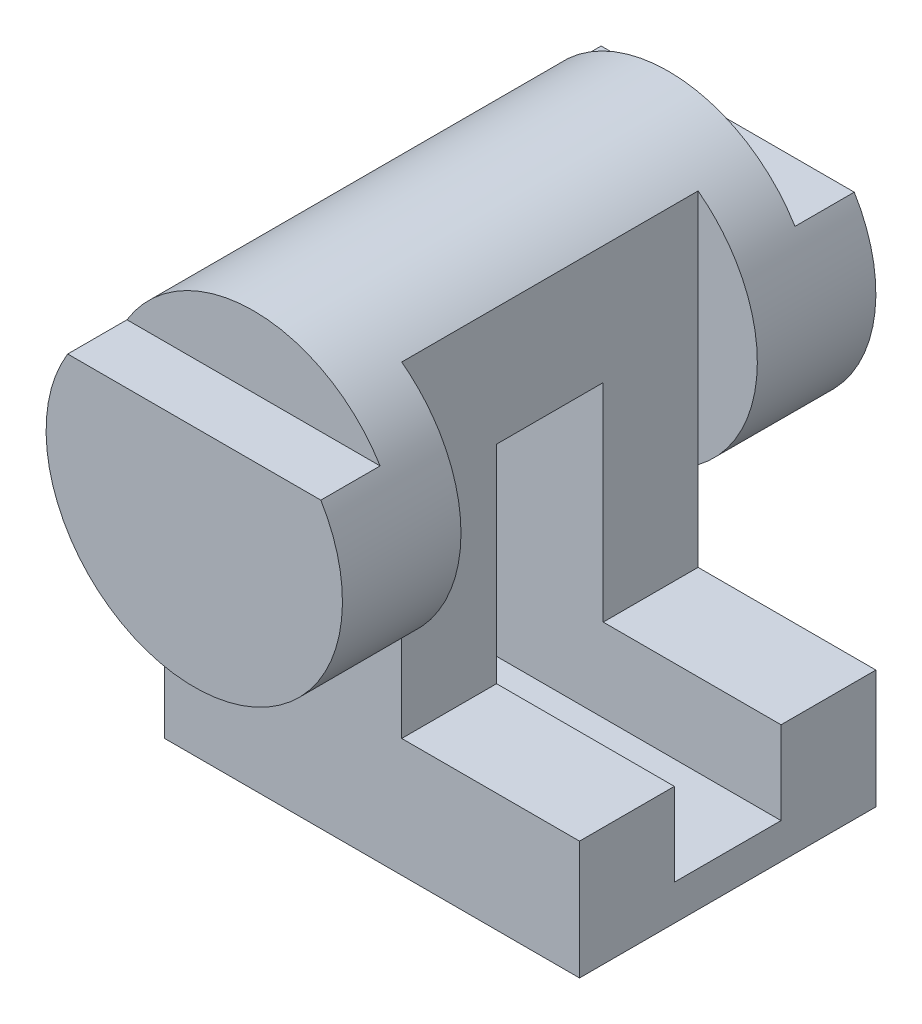
ISO-10303-21;
HEADER;
FILE_DESCRIPTION(('STEP AP214'),'2;1');
FILE_NAME('part.step','',(''),(''),'','','');
FILE_SCHEMA(('AUTOMOTIVE_DESIGN { 1 0 10303 214 1 1 1 1 }'));
ENDSEC;
DATA;
#1=APPLICATION_CONTEXT('core data for automotive mechanical design processes');
#2=APPLICATION_PROTOCOL_DEFINITION('international standard','automotive_design',2000,#1);
#3=PRODUCT_CONTEXT('',#1,'mechanical');
#4=PRODUCT('Part','Part','',(#3));
#5=PRODUCT_RELATED_PRODUCT_CATEGORY('part','',(#4));
#6=PRODUCT_DEFINITION_FORMATION('','',#4);
#7=PRODUCT_DEFINITION_CONTEXT('part definition',#1,'design');
#8=PRODUCT_DEFINITION('design','',#6,#7);
#9=PRODUCT_DEFINITION_SHAPE('','',#8);
#10=(LENGTH_UNIT() NAMED_UNIT(*) SI_UNIT(.MILLI.,.METRE.));
#11=(NAMED_UNIT(*) PLANE_ANGLE_UNIT() SI_UNIT($,.RADIAN.));
#12=(NAMED_UNIT(*) SI_UNIT($,.STERADIAN.) SOLID_ANGLE_UNIT());
#13=UNCERTAINTY_MEASURE_WITH_UNIT(LENGTH_MEASURE(1.E-05),#10,'distance_accuracy_value','');
#14=(GEOMETRIC_REPRESENTATION_CONTEXT(3) GLOBAL_UNCERTAINTY_ASSIGNED_CONTEXT((#13)) GLOBAL_UNIT_ASSIGNED_CONTEXT((#10,
#11,#12)) REPRESENTATION_CONTEXT('',''));
#15=CARTESIAN_POINT('',(0.,0.,0.));
#16=DIRECTION('',(0.,0.,1.));
#17=DIRECTION('',(1.,0.,0.));
#18=AXIS2_PLACEMENT_3D('',#15,#16,#17);
#19=CARTESIAN_POINT('',(20.,0.,25.));
#20=DIRECTION('',(0.,0.,-1.));
#21=DIRECTION('',(-1.,0.,0.));
#22=AXIS2_PLACEMENT_3D('',#19,#20,#21);
#23=PLANE('',#22);
#24=CARTESIAN_POINT('',(-25.,55.,25.));
#25=DIRECTION('',(0.,0.,1.));
#26=DIRECTION('',(1.,0.,0.));
#27=AXIS2_PLACEMENT_3D('',#24,#25,#26);
#28=CIRCLE('',#27,25.);
#29=CARTESIAN_POINT('',(-50.,55.,25.));
#30=VERTEX_POINT('',#29);
#31=CARTESIAN_POINT('',(-10.,35.,25.));
#32=VERTEX_POINT('',#31);
#33=EDGE_CURVE('E57',#30,#32,#28,.T.);
#34=ORIENTED_EDGE('',*,*,#33,.F.);
#35=DIRECTION('',(0.,1.,0.));
#36=VECTOR('',#35,1.);
#37=CARTESIAN_POINT('',(-50.,0.,25.));
#38=LINE('',#37,#36);
#39=CARTESIAN_POINT('',(-50.,0.,25.));
#40=VERTEX_POINT('',#39);
#41=EDGE_CURVE('E246',#40,#30,#38,.T.);
#42=ORIENTED_EDGE('',*,*,#41,.F.);
#43=DIRECTION('',(-1.,0.,0.));
#44=VECTOR('',#43,1.);
#45=CARTESIAN_POINT('',(20.,0.,25.));
#46=LINE('',#45,#44);
#47=CARTESIAN_POINT('',(20.,0.,25.));
#48=VERTEX_POINT('',#47);
#49=EDGE_CURVE('E283',#48,#40,#46,.T.);
#50=ORIENTED_EDGE('',*,*,#49,.F.);
#51=DIRECTION('',(0.,-1.,0.));
#52=VECTOR('',#51,1.);
#53=CARTESIAN_POINT('',(20.,0.,25.));
#54=LINE('',#53,#52);
#55=CARTESIAN_POINT('',(20.,20.,25.));
#56=VERTEX_POINT('',#55);
#57=EDGE_CURVE('E261',#56,#48,#54,.T.);
#58=ORIENTED_EDGE('',*,*,#57,.F.);
#59=DIRECTION('',(-1.,0.,0.));
#60=VECTOR('',#59,1.);
#61=CARTESIAN_POINT('',(20.,20.,25.));
#62=LINE('',#61,#60);
#63=CARTESIAN_POINT('',(-10.,20.,25.));
#64=VERTEX_POINT('',#63);
#65=EDGE_CURVE('E284',#56,#64,#62,.T.);
#66=ORIENTED_EDGE('',*,*,#65,.T.);
#67=DIRECTION('',(0.,-1.,0.));
#68=VECTOR('',#67,1.);
#69=CARTESIAN_POINT('',(-10.,20.,25.));
#70=LINE('',#69,#68);
#71=EDGE_CURVE('E212',#32,#64,#70,.T.);
#72=ORIENTED_EDGE('',*,*,#71,.F.);
#73=EDGE_LOOP('',(#34,#42,#50,#58,#66,#72));
#74=FACE_BOUND('',#73,.T.);
#75=ADVANCED_FACE('F50',(#74),#23,.F.);
#76=CARTESIAN_POINT('',(20.,20.,-25.));
#77=DIRECTION('',(0.,0.,1.));
#78=DIRECTION('',(1.,0.,0.));
#79=AXIS2_PLACEMENT_3D('',#76,#77,#78);
#80=PLANE('',#79);
#81=CARTESIAN_POINT('',(-25.,55.,-25.));
#82=DIRECTION('',(0.,0.,-1.));
#83=DIRECTION('',(-1.,0.,0.));
#84=AXIS2_PLACEMENT_3D('',#81,#82,#83);
#85=CIRCLE('',#84,25.);
#86=CARTESIAN_POINT('',(-10.,35.,-25.));
#87=VERTEX_POINT('',#86);
#88=CARTESIAN_POINT('',(-50.,55.,-25.));
#89=VERTEX_POINT('',#88);
#90=EDGE_CURVE('E11',#87,#89,#85,.T.);
#91=ORIENTED_EDGE('',*,*,#90,.F.);
#92=DIRECTION('',(0.,1.,0.));
#93=VECTOR('',#92,1.);
#94=CARTESIAN_POINT('',(-10.,20.,-25.));
#95=LINE('',#94,#93);
#96=CARTESIAN_POINT('',(-10.,20.,-25.));
#97=VERTEX_POINT('',#96);
#98=EDGE_CURVE('E217',#97,#87,#95,.T.);
#99=ORIENTED_EDGE('',*,*,#98,.F.);
#100=DIRECTION('',(-1.,0.,0.));
#101=VECTOR('',#100,1.);
#102=CARTESIAN_POINT('',(20.,20.,-25.));
#103=LINE('',#102,#101);
#104=CARTESIAN_POINT('',(20.,20.,-25.));
#105=VERTEX_POINT('',#104);
#106=EDGE_CURVE('E276',#105,#97,#103,.T.);
#107=ORIENTED_EDGE('',*,*,#106,.F.);
#108=DIRECTION('',(0.,1.,0.));
#109=VECTOR('',#108,1.);
#110=CARTESIAN_POINT('',(20.,20.,-25.));
#111=LINE('',#110,#109);
#112=CARTESIAN_POINT('',(20.,0.,-25.));
#113=VERTEX_POINT('',#112);
#114=EDGE_CURVE('E264',#113,#105,#111,.T.);
#115=ORIENTED_EDGE('',*,*,#114,.F.);
#116=DIRECTION('',(-1.,0.,0.));
#117=VECTOR('',#116,1.);
#118=CARTESIAN_POINT('',(20.,0.,-25.));
#119=LINE('',#118,#117);
#120=CARTESIAN_POINT('',(-50.,0.,-25.));
#121=VERTEX_POINT('',#120);
#122=EDGE_CURVE('E281',#113,#121,#119,.T.);
#123=ORIENTED_EDGE('',*,*,#122,.T.);
#124=DIRECTION('',(0.,1.,0.));
#125=VECTOR('',#124,1.);
#126=CARTESIAN_POINT('',(-50.,0.,-25.));
#127=LINE('',#126,#125);
#128=EDGE_CURVE('E241',#121,#89,#127,.T.);
#129=ORIENTED_EDGE('',*,*,#128,.T.);
#130=EDGE_LOOP('',(#91,#99,#107,#115,#123,#129));
#131=FACE_BOUND('',#130,.T.);
#132=ADVANCED_FACE('F332',(#131),#80,.F.);
#133=CARTESIAN_POINT('',(20.,20.,9.));
#134=DIRECTION('',(0.,0.,1.));
#135=DIRECTION('',(0.,-1.,0.));
#136=AXIS2_PLACEMENT_3D('',#133,#134,#135);
#137=PLANE('',#136);
#138=DIRECTION('',(0.,-1.,0.));
#139=VECTOR('',#138,1.);
#140=CARTESIAN_POINT('',(-10.,20.,9.));
#141=LINE('',#140,#139);
#142=CARTESIAN_POINT('',(-10.,55.,9.));
#143=VERTEX_POINT('',#142);
#144=CARTESIAN_POINT('',(-10.,20.,9.00000000000001));
#145=VERTEX_POINT('',#144);
#146=EDGE_CURVE('E223',#143,#145,#141,.T.);
#147=ORIENTED_EDGE('',*,*,#146,.T.);
#148=DIRECTION('',(-1.,0.,0.));
#149=VECTOR('',#148,1.);
#150=CARTESIAN_POINT('',(20.,20.,9.));
#151=LINE('',#150,#149);
#152=CARTESIAN_POINT('',(20.,20.,9.));
#153=VERTEX_POINT('',#152);
#154=EDGE_CURVE('E290',#153,#145,#151,.T.);
#155=ORIENTED_EDGE('',*,*,#154,.F.);
#156=DIRECTION('',(0.,1.,0.));
#157=VECTOR('',#156,1.);
#158=CARTESIAN_POINT('',(20.,20.,9.));
#159=LINE('',#158,#157);
#160=CARTESIAN_POINT('',(20.,5.99999999999999,9.));
#161=VERTEX_POINT('',#160);
#162=EDGE_CURVE('E257',#161,#153,#159,.T.);
#163=ORIENTED_EDGE('',*,*,#162,.F.);
#164=DIRECTION('',(-1.,0.,0.));
#165=VECTOR('',#164,1.);
#166=CARTESIAN_POINT('',(20.,5.99999999999999,9.));
#167=LINE('',#166,#165);
#168=CARTESIAN_POINT('',(-50.,5.99999999999999,9.));
#169=VERTEX_POINT('',#168);
#170=EDGE_CURVE('E271',#161,#169,#167,.T.);
#171=ORIENTED_EDGE('',*,*,#170,.T.);
#172=DIRECTION('',(0.,1.,0.));
#173=VECTOR('',#172,1.);
#174=CARTESIAN_POINT('',(-50.,0.,9.));
#175=LINE('',#174,#173);
#176=CARTESIAN_POINT('',(-50.,55.,9.));
#177=VERTEX_POINT('',#176);
#178=EDGE_CURVE('E251',#169,#177,#175,.T.);
#179=ORIENTED_EDGE('',*,*,#178,.T.);
#180=DIRECTION('',(1.,0.,0.));
#181=VECTOR('',#180,1.);
#182=CARTESIAN_POINT('',(-50.,55.,9.));
#183=LINE('',#182,#181);
#184=EDGE_CURVE('E235',#177,#143,#183,.T.);
#185=ORIENTED_EDGE('',*,*,#184,.T.);
#186=EDGE_LOOP('',(#147,#155,#163,#171,#179,#185));
#187=FACE_BOUND('',#186,.T.);
#188=ADVANCED_FACE('F47',(#187),#137,.F.);
#189=CARTESIAN_POINT('',(20.,20.,25.));
#190=DIRECTION('',(0.,-1.,0.));
#191=DIRECTION('',(0.,0.,-1.));
#192=AXIS2_PLACEMENT_3D('',#189,#190,#191);
#193=PLANE('',#192);
#194=ORIENTED_EDGE('',*,*,#154,.T.);
#195=DIRECTION('',(0.,0.,-1.));
#196=VECTOR('',#195,1.);
#197=CARTESIAN_POINT('',(-10.,20.,25.));
#198=LINE('',#197,#196);
#199=EDGE_CURVE('E213',#64,#145,#198,.T.);
#200=ORIENTED_EDGE('',*,*,#199,.F.);
#201=ORIENTED_EDGE('',*,*,#65,.F.);
#202=DIRECTION('',(0.,0.,1.));
#203=VECTOR('',#202,1.);
#204=CARTESIAN_POINT('',(20.,20.,25.));
#205=LINE('',#204,#203);
#206=EDGE_CURVE('E256',#153,#56,#205,.T.);
#207=ORIENTED_EDGE('',*,*,#206,.F.);
#208=EDGE_LOOP('',(#194,#200,#201,#207));
#209=FACE_BOUND('',#208,.T.);
#210=ADVANCED_FACE('F345',(#209),#193,.F.);
#211=CARTESIAN_POINT('',(20.,0.,-25.));
#212=DIRECTION('',(0.,1.,0.));
#213=DIRECTION('',(0.,0.,1.));
#214=AXIS2_PLACEMENT_3D('',#211,#212,#213);
#215=PLANE('',#214);
#216=ORIENTED_EDGE('',*,*,#49,.T.);
#217=DIRECTION('',(0.,0.,1.));
#218=VECTOR('',#217,1.);
#219=CARTESIAN_POINT('',(-50.,0.,0.));
#220=LINE('',#219,#218);
#221=EDGE_CURVE('E243',#121,#40,#220,.T.);
#222=ORIENTED_EDGE('',*,*,#221,.F.);
#223=ORIENTED_EDGE('',*,*,#122,.F.);
#224=DIRECTION('',(0.,0.,-1.));
#225=VECTOR('',#224,1.);
#226=CARTESIAN_POINT('',(20.,0.,-25.));
#227=LINE('',#226,#225);
#228=EDGE_CURVE('E263',#48,#113,#227,.T.);
#229=ORIENTED_EDGE('',*,*,#228,.F.);
#230=EDGE_LOOP('',(#216,#222,#223,#229));
#231=FACE_BOUND('',#230,.T.);
#232=ADVANCED_FACE('F342',(#231),#215,.F.);
#233=CARTESIAN_POINT('',(20.,20.,-9.));
#234=DIRECTION('',(0.,-1.,0.));
#235=DIRECTION('',(0.,0.,-1.));
#236=AXIS2_PLACEMENT_3D('',#233,#234,#235);
#237=PLANE('',#236);
#238=ORIENTED_EDGE('',*,*,#106,.T.);
#239=CARTESIAN_POINT('',(-10.,20.,-9.));
#240=VERTEX_POINT('',#239);
#241=EDGE_CURVE('E211',#240,#97,#198,.T.);
#242=ORIENTED_EDGE('',*,*,#241,.F.);
#243=DIRECTION('',(-1.,0.,0.));
#244=VECTOR('',#243,1.);
#245=CARTESIAN_POINT('',(20.,20.,-9.));
#246=LINE('',#245,#244);
#247=CARTESIAN_POINT('',(20.,20.,-9.));
#248=VERTEX_POINT('',#247);
#249=EDGE_CURVE('E280',#248,#240,#246,.T.);
#250=ORIENTED_EDGE('',*,*,#249,.F.);
#251=DIRECTION('',(0.,0.,1.));
#252=VECTOR('',#251,1.);
#253=CARTESIAN_POINT('',(20.,20.,-9.));
#254=LINE('',#253,#252);
#255=EDGE_CURVE('E270',#105,#248,#254,.T.);
#256=ORIENTED_EDGE('',*,*,#255,.F.);
#257=EDGE_LOOP('',(#238,#242,#250,#256));
#258=FACE_BOUND('',#257,.T.);
#259=ADVANCED_FACE('F347',(#258),#237,.F.);
#260=CARTESIAN_POINT('',(20.,5.99999999999999,-9.));
#261=DIRECTION('',(0.,0.,-1.));
#262=DIRECTION('',(-1.,0.,0.));
#263=AXIS2_PLACEMENT_3D('',#260,#261,#262);
#264=PLANE('',#263);
#265=ORIENTED_EDGE('',*,*,#249,.T.);
#266=DIRECTION('',(0.,1.,0.));
#267=VECTOR('',#266,1.);
#268=CARTESIAN_POINT('',(-10.,5.99999999999999,-9.));
#269=LINE('',#268,#267);
#270=CARTESIAN_POINT('',(-10.,55.,-9.));
#271=VERTEX_POINT('',#270);
#272=EDGE_CURVE('E225',#240,#271,#269,.T.);
#273=ORIENTED_EDGE('',*,*,#272,.T.);
#274=DIRECTION('',(1.,0.,0.));
#275=VECTOR('',#274,1.);
#276=CARTESIAN_POINT('',(-50.,55.,-9.));
#277=LINE('',#276,#275);
#278=CARTESIAN_POINT('',(-50.,55.,-9.));
#279=VERTEX_POINT('',#278);
#280=EDGE_CURVE('E233',#279,#271,#277,.T.);
#281=ORIENTED_EDGE('',*,*,#280,.F.);
#282=DIRECTION('',(0.,1.,0.));
#283=VECTOR('',#282,1.);
#284=CARTESIAN_POINT('',(-50.,0.,-9.));
#285=LINE('',#284,#283);
#286=CARTESIAN_POINT('',(-50.,5.99999999999999,-9.));
#287=VERTEX_POINT('',#286);
#288=EDGE_CURVE('E255',#287,#279,#285,.T.);
#289=ORIENTED_EDGE('',*,*,#288,.F.);
#290=DIRECTION('',(-1.,0.,0.));
#291=VECTOR('',#290,1.);
#292=CARTESIAN_POINT('',(20.,5.99999999999999,-9.));
#293=LINE('',#292,#291);
#294=CARTESIAN_POINT('',(20.,5.99999999999999,-9.));
#295=VERTEX_POINT('',#294);
#296=EDGE_CURVE('E273',#295,#287,#293,.T.);
#297=ORIENTED_EDGE('',*,*,#296,.F.);
#298=DIRECTION('',(0.,-1.,0.));
#299=VECTOR('',#298,1.);
#300=CARTESIAN_POINT('',(20.,5.99999999999999,-9.));
#301=LINE('',#300,#299);
#302=EDGE_CURVE('E266',#248,#295,#301,.T.);
#303=ORIENTED_EDGE('',*,*,#302,.F.);
#304=EDGE_LOOP('',(#265,#273,#281,#289,#297,#303));
#305=FACE_BOUND('',#304,.T.);
#306=ADVANCED_FACE('F384',(#305),#264,.F.);
#307=CARTESIAN_POINT('',(20.,5.99999999999999,9.));
#308=DIRECTION('',(0.,-1.,0.));
#309=DIRECTION('',(0.,0.,-1.));
#310=AXIS2_PLACEMENT_3D('',#307,#308,#309);
#311=PLANE('',#310);
#312=ORIENTED_EDGE('',*,*,#296,.T.);
#313=DIRECTION('',(0.,0.,-1.));
#314=VECTOR('',#313,1.);
#315=CARTESIAN_POINT('',(-50.,5.99999999999999,0.));
#316=LINE('',#315,#314);
#317=EDGE_CURVE('E248',#169,#287,#316,.T.);
#318=ORIENTED_EDGE('',*,*,#317,.F.);
#319=ORIENTED_EDGE('',*,*,#170,.F.);
#320=DIRECTION('',(0.,0.,1.));
#321=VECTOR('',#320,1.);
#322=CARTESIAN_POINT('',(20.,5.99999999999999,9.));
#323=LINE('',#322,#321);
#324=EDGE_CURVE('E272',#295,#161,#323,.T.);
#325=ORIENTED_EDGE('',*,*,#324,.F.);
#326=EDGE_LOOP('',(#312,#318,#319,#325));
#327=FACE_BOUND('',#326,.T.);
#328=ADVANCED_FACE('F362',(#327),#311,.F.);
#329=CARTESIAN_POINT('',(20.,0.,0.));
#330=DIRECTION('',(1.,0.,0.));
#331=DIRECTION('',(0.,0.,-1.));
#332=AXIS2_PLACEMENT_3D('',#329,#330,#331);
#333=PLANE('',#332);
#334=ORIENTED_EDGE('',*,*,#162,.T.);
#335=ORIENTED_EDGE('',*,*,#206,.T.);
#336=ORIENTED_EDGE('',*,*,#57,.T.);
#337=ORIENTED_EDGE('',*,*,#228,.T.);
#338=ORIENTED_EDGE('',*,*,#114,.T.);
#339=ORIENTED_EDGE('',*,*,#255,.T.);
#340=ORIENTED_EDGE('',*,*,#302,.T.);
#341=ORIENTED_EDGE('',*,*,#324,.T.);
#342=EDGE_LOOP('',(#334,#335,#336,#337,#338,#339,#340,#341));
#343=FACE_BOUND('',#342,.T.);
#344=ADVANCED_FACE('F356',(#343),#333,.T.);
#345=CARTESIAN_POINT('',(-50.,0.,0.));
#346=DIRECTION('',(-1.,0.,0.));
#347=DIRECTION('',(0.,0.,1.));
#348=AXIS2_PLACEMENT_3D('',#345,#346,#347);
#349=PLANE('',#348);
#350=DIRECTION('',(0.,0.,1.));
#351=VECTOR('',#350,1.);
#352=CARTESIAN_POINT('',(-50.,55.,-25.));
#353=LINE('',#352,#351);
#354=EDGE_CURVE('E238',#89,#279,#353,.T.);
#355=ORIENTED_EDGE('',*,*,#354,.F.);
#356=ORIENTED_EDGE('',*,*,#128,.F.);
#357=ORIENTED_EDGE('',*,*,#221,.T.);
#358=ORIENTED_EDGE('',*,*,#41,.T.);
#359=EDGE_CURVE('E232',#177,#30,#353,.T.);
#360=ORIENTED_EDGE('',*,*,#359,.F.);
#361=ORIENTED_EDGE('',*,*,#178,.F.);
#362=ORIENTED_EDGE('',*,*,#317,.T.);
#363=ORIENTED_EDGE('',*,*,#288,.T.);
#364=EDGE_LOOP('',(#355,#356,#357,#358,#360,#361,#362,#363));
#365=FACE_BOUND('',#364,.T.);
#366=ADVANCED_FACE('F369',(#365),#349,.T.);
#367=CARTESIAN_POINT('',(-25.,55.,-25.));
#368=DIRECTION('',(0.,0.,1.));
#369=DIRECTION('',(1.,0.,0.));
#370=AXIS2_PLACEMENT_3D('',#367,#368,#369);
#371=CYLINDRICAL_SURFACE('',#370,25.);
#372=DIRECTION('',(0.,0.,-1.));
#373=VECTOR('',#372,1.);
#374=CARTESIAN_POINT('',(-3.64584349593737,68.,-35.));
#375=LINE('',#374,#373);
#376=CARTESIAN_POINT('',(-3.64584349593737,68.,-35.));
#377=VERTEX_POINT('',#376);
#378=CARTESIAN_POINT('',(-3.64584349593738,68.,-45.));
#379=VERTEX_POINT('',#378);
#380=EDGE_CURVE('E63',#377,#379,#375,.T.);
#381=ORIENTED_EDGE('',*,*,#380,.F.);
#382=CARTESIAN_POINT('',(-25.,55.,-35.));
#383=DIRECTION('',(0.,0.,-1.));
#384=DIRECTION('',(-1.,0.,0.));
#385=AXIS2_PLACEMENT_3D('',#382,#383,#384);
#386=CIRCLE('',#385,25.);
#387=CARTESIAN_POINT('',(-46.3541565040626,68.,-35.));
#388=VERTEX_POINT('',#387);
#389=EDGE_CURVE('E171',#388,#377,#386,.T.);
#390=ORIENTED_EDGE('',*,*,#389,.F.);
#391=DIRECTION('',(0.,0.,-1.));
#392=VECTOR('',#391,1.);
#393=CARTESIAN_POINT('',(-46.3541565040626,68.,-35.));
#394=LINE('',#393,#392);
#395=CARTESIAN_POINT('',(-46.3541565040626,68.,-45.));
#396=VERTEX_POINT('',#395);
#397=EDGE_CURVE('E177',#388,#396,#394,.T.);
#398=ORIENTED_EDGE('',*,*,#397,.T.);
#399=CARTESIAN_POINT('',(-25.,55.,-45.));
#400=DIRECTION('',(0.,0.,-1.));
#401=DIRECTION('',(-1.,0.,0.));
#402=AXIS2_PLACEMENT_3D('',#399,#400,#401);
#403=CIRCLE('',#402,25.);
#404=EDGE_CURVE('E184',#379,#396,#403,.T.);
#405=ORIENTED_EDGE('',*,*,#404,.F.);
#406=EDGE_LOOP('',(#381,#390,#398,#405));
#407=FACE_BOUND('',#406,.T.);
#408=DIRECTION('',(0.,0.,1.));
#409=VECTOR('',#408,1.);
#410=CARTESIAN_POINT('',(-3.64584349593737,68.,35.));
#411=LINE('',#410,#409);
#412=CARTESIAN_POINT('',(-3.64584349593737,68.,35.));
#413=VERTEX_POINT('',#412);
#414=CARTESIAN_POINT('',(-3.64584349593737,68.,45.));
#415=VERTEX_POINT('',#414);
#416=EDGE_CURVE('E200',#413,#415,#411,.T.);
#417=ORIENTED_EDGE('',*,*,#416,.T.);
#418=CARTESIAN_POINT('',(-25.,55.,45.));
#419=DIRECTION('',(0.,0.,1.));
#420=DIRECTION('',(1.,0.,0.));
#421=AXIS2_PLACEMENT_3D('',#418,#419,#420);
#422=CIRCLE('',#421,25.);
#423=CARTESIAN_POINT('',(-46.3541565040626,68.,45.));
#424=VERTEX_POINT('',#423);
#425=EDGE_CURVE('E201',#424,#415,#422,.T.);
#426=ORIENTED_EDGE('',*,*,#425,.F.);
#427=DIRECTION('',(0.,0.,1.));
#428=VECTOR('',#427,1.);
#429=CARTESIAN_POINT('',(-46.3541565040626,68.,35.));
#430=LINE('',#429,#428);
#431=CARTESIAN_POINT('',(-46.3541565040626,68.,35.));
#432=VERTEX_POINT('',#431);
#433=EDGE_CURVE('E74',#432,#424,#430,.T.);
#434=ORIENTED_EDGE('',*,*,#433,.F.);
#435=CARTESIAN_POINT('',(-25.,55.,35.));
#436=DIRECTION('',(0.,0.,1.));
#437=DIRECTION('',(1.,0.,0.));
#438=AXIS2_PLACEMENT_3D('',#435,#436,#437);
#439=CIRCLE('',#438,25.);
#440=EDGE_CURVE('E192',#413,#432,#439,.T.);
#441=ORIENTED_EDGE('',*,*,#440,.F.);
#442=EDGE_LOOP('',(#417,#426,#434,#441));
#443=FACE_BOUND('',#442,.T.);
#444=DIRECTION('',(0.,0.,1.));
#445=VECTOR('',#444,1.);
#446=CARTESIAN_POINT('',(-10.,75.,-25.));
#447=LINE('',#446,#445);
#448=CARTESIAN_POINT('',(-10.,75.,-25.));
#449=VERTEX_POINT('',#448);
#450=CARTESIAN_POINT('',(-10.,75.,25.));
#451=VERTEX_POINT('',#450);
#452=EDGE_CURVE('E210',#449,#451,#447,.T.);
#453=ORIENTED_EDGE('',*,*,#452,.F.);
#454=EDGE_CURVE('E59',#449,#87,#85,.T.);
#455=ORIENTED_EDGE('',*,*,#454,.T.);
#456=ORIENTED_EDGE('',*,*,#90,.T.);
#457=ORIENTED_EDGE('',*,*,#354,.T.);
#458=DIRECTION('',(0.,0.,1.));
#459=VECTOR('',#458,1.);
#460=CARTESIAN_POINT('',(-50.,55.,9.));
#461=LINE('',#460,#459);
#462=EDGE_CURVE('E226',#279,#177,#461,.T.);
#463=ORIENTED_EDGE('',*,*,#462,.T.);
#464=ORIENTED_EDGE('',*,*,#359,.T.);
#465=ORIENTED_EDGE('',*,*,#33,.T.);
#466=EDGE_CURVE('E202',#32,#451,#28,.T.);
#467=ORIENTED_EDGE('',*,*,#466,.T.);
#468=EDGE_LOOP('',(#453,#455,#456,#457,#463,#464,#465,#467));
#469=FACE_BOUND('',#468,.T.);
#470=ADVANCED_FACE('F185',(#407,#443,#469),#371,.T.);
#471=CARTESIAN_POINT('',(-50.,55.,9.));
#472=DIRECTION('',(0.,1.,0.));
#473=DIRECTION('',(0.,0.,1.));
#474=AXIS2_PLACEMENT_3D('',#471,#472,#473);
#475=PLANE('',#474);
#476=ORIENTED_EDGE('',*,*,#280,.T.);
#477=DIRECTION('',(0.,0.,1.));
#478=VECTOR('',#477,1.);
#479=CARTESIAN_POINT('',(-10.,55.,9.));
#480=LINE('',#479,#478);
#481=EDGE_CURVE('E51',#271,#143,#480,.T.);
#482=ORIENTED_EDGE('',*,*,#481,.T.);
#483=ORIENTED_EDGE('',*,*,#184,.F.);
#484=ORIENTED_EDGE('',*,*,#462,.F.);
#485=EDGE_LOOP('',(#476,#482,#483,#484));
#486=FACE_BOUND('',#485,.T.);
#487=ADVANCED_FACE('F387',(#486),#475,.F.);
#488=CARTESIAN_POINT('',(-10.,0.,0.));
#489=DIRECTION('',(-1.,0.,0.));
#490=DIRECTION('',(0.,0.,1.));
#491=AXIS2_PLACEMENT_3D('',#488,#489,#490);
#492=PLANE('',#491);
#493=ORIENTED_EDGE('',*,*,#481,.F.);
#494=ORIENTED_EDGE('',*,*,#272,.F.);
#495=ORIENTED_EDGE('',*,*,#241,.T.);
#496=ORIENTED_EDGE('',*,*,#98,.T.);
#497=EDGE_CURVE('E218',#87,#449,#95,.T.);
#498=ORIENTED_EDGE('',*,*,#497,.T.);
#499=ORIENTED_EDGE('',*,*,#452,.T.);
#500=EDGE_CURVE('E215',#451,#32,#70,.T.);
#501=ORIENTED_EDGE('',*,*,#500,.T.);
#502=ORIENTED_EDGE('',*,*,#71,.T.);
#503=ORIENTED_EDGE('',*,*,#199,.T.);
#504=ORIENTED_EDGE('',*,*,#146,.F.);
#505=EDGE_LOOP('',(#493,#494,#495,#496,#498,#499,#501,#502,#503,#504));
#506=FACE_BOUND('',#505,.T.);
#507=ADVANCED_FACE('F309',(#506),#492,.F.);
#508=CARTESIAN_POINT('',(-25.,55.,45.));
#509=DIRECTION('',(0.,0.,1.));
#510=DIRECTION('',(1.,0.,0.));
#511=AXIS2_PLACEMENT_3D('',#508,#509,#510);
#512=PLANE('',#511);
#513=DIRECTION('',(1.,0.,0.));
#514=VECTOR('',#513,1.);
#515=CARTESIAN_POINT('',(-46.3541565040626,68.,45.));
#516=LINE('',#515,#514);
#517=EDGE_CURVE('E190',#424,#415,#516,.T.);
#518=ORIENTED_EDGE('',*,*,#517,.F.);
#519=ORIENTED_EDGE('',*,*,#425,.T.);
#520=EDGE_LOOP('',(#518,#519));
#521=FACE_BOUND('',#520,.T.);
#522=ADVANCED_FACE('F395',(#521),#512,.T.);
#523=CARTESIAN_POINT('',(-25.,55.,25.));
#524=DIRECTION('',(0.,0.,1.));
#525=DIRECTION('',(1.,0.,0.));
#526=AXIS2_PLACEMENT_3D('',#523,#524,#525);
#527=PLANE('',#526);
#528=ORIENTED_EDGE('',*,*,#500,.F.);
#529=ORIENTED_EDGE('',*,*,#466,.F.);
#530=EDGE_LOOP('',(#528,#529));
#531=FACE_BOUND('',#530,.T.);
#532=ADVANCED_FACE('F307',(#531),#527,.F.);
#533=CARTESIAN_POINT('',(-25.,55.,-45.));
#534=DIRECTION('',(0.,0.,-1.));
#535=DIRECTION('',(-1.,0.,0.));
#536=AXIS2_PLACEMENT_3D('',#533,#534,#535);
#537=PLANE('',#536);
#538=DIRECTION('',(-1.,0.,0.));
#539=VECTOR('',#538,1.);
#540=CARTESIAN_POINT('',(-3.64584349593737,68.,-45.));
#541=LINE('',#540,#539);
#542=EDGE_CURVE('E176',#379,#396,#541,.T.);
#543=ORIENTED_EDGE('',*,*,#542,.F.);
#544=ORIENTED_EDGE('',*,*,#404,.T.);
#545=EDGE_LOOP('',(#543,#544));
#546=FACE_BOUND('',#545,.T.);
#547=ADVANCED_FACE('F320',(#546),#537,.T.);
#548=CARTESIAN_POINT('',(-25.,55.,-25.));
#549=DIRECTION('',(0.,0.,-1.));
#550=DIRECTION('',(-1.,0.,0.));
#551=AXIS2_PLACEMENT_3D('',#548,#549,#550);
#552=PLANE('',#551);
#553=ORIENTED_EDGE('',*,*,#497,.F.);
#554=ORIENTED_EDGE('',*,*,#454,.F.);
#555=EDGE_LOOP('',(#553,#554));
#556=FACE_BOUND('',#555,.T.);
#557=ADVANCED_FACE('F313',(#556),#552,.F.);
#558=CARTESIAN_POINT('',(-46.3541565040626,68.,35.));
#559=DIRECTION('',(0.,-1.,0.));
#560=DIRECTION('',(0.,0.,-1.));
#561=AXIS2_PLACEMENT_3D('',#558,#559,#560);
#562=PLANE('',#561);
#563=ORIENTED_EDGE('',*,*,#517,.T.);
#564=ORIENTED_EDGE('',*,*,#416,.F.);
#565=DIRECTION('',(1.,0.,0.));
#566=VECTOR('',#565,1.);
#567=CARTESIAN_POINT('',(-46.3541565040626,68.,35.));
#568=LINE('',#567,#566);
#569=EDGE_CURVE('E194',#432,#413,#568,.T.);
#570=ORIENTED_EDGE('',*,*,#569,.F.);
#571=ORIENTED_EDGE('',*,*,#433,.T.);
#572=EDGE_LOOP('',(#563,#564,#570,#571));
#573=FACE_BOUND('',#572,.T.);
#574=ADVANCED_FACE('F317',(#573),#562,.F.);
#575=CARTESIAN_POINT('',(-25.,55.,35.));
#576=DIRECTION('',(0.,0.,1.));
#577=DIRECTION('',(1.,0.,0.));
#578=AXIS2_PLACEMENT_3D('',#575,#576,#577);
#579=PLANE('',#578);
#580=ORIENTED_EDGE('',*,*,#440,.T.);
#581=ORIENTED_EDGE('',*,*,#569,.T.);
#582=EDGE_LOOP('',(#580,#581));
#583=FACE_BOUND('',#582,.T.);
#584=ADVANCED_FACE('F321',(#583),#579,.T.);
#585=CARTESIAN_POINT('',(-3.64584349593737,68.,-35.));
#586=DIRECTION('',(0.,-1.,0.));
#587=DIRECTION('',(0.,0.,-1.));
#588=AXIS2_PLACEMENT_3D('',#585,#586,#587);
#589=PLANE('',#588);
#590=ORIENTED_EDGE('',*,*,#542,.T.);
#591=ORIENTED_EDGE('',*,*,#397,.F.);
#592=DIRECTION('',(-1.,0.,0.));
#593=VECTOR('',#592,1.);
#594=CARTESIAN_POINT('',(-3.64584349593737,68.,-35.));
#595=LINE('',#594,#593);
#596=EDGE_CURVE('E173',#377,#388,#595,.T.);
#597=ORIENTED_EDGE('',*,*,#596,.F.);
#598=ORIENTED_EDGE('',*,*,#380,.T.);
#599=EDGE_LOOP('',(#590,#591,#597,#598));
#600=FACE_BOUND('',#599,.T.);
#601=ADVANCED_FACE('F178',(#600),#589,.F.);
#602=CARTESIAN_POINT('',(-25.,55.,-35.));
#603=DIRECTION('',(0.,0.,-1.));
#604=DIRECTION('',(-1.,0.,0.));
#605=AXIS2_PLACEMENT_3D('',#602,#603,#604);
#606=PLANE('',#605);
#607=ORIENTED_EDGE('',*,*,#389,.T.);
#608=ORIENTED_EDGE('',*,*,#596,.T.);
#609=EDGE_LOOP('',(#607,#608));
#610=FACE_BOUND('',#609,.T.);
#611=ADVANCED_FACE('F175',(#610),#606,.T.);
#612=CLOSED_SHELL('',(#75,#132,#188,#210,#232,#259,#306,#328,#344,#366,#470,#487,#507,#522,#532,
#547,#557,#574,#584,#601,#611));
#613=MANIFOLD_SOLID_BREP('B2',#612);
#614=ADVANCED_BREP_SHAPE_REPRESENTATION('',(#18,#613),#14);
#615=SHAPE_DEFINITION_REPRESENTATION(#9,#614);
ENDSEC;
END-ISO-10303-21;
